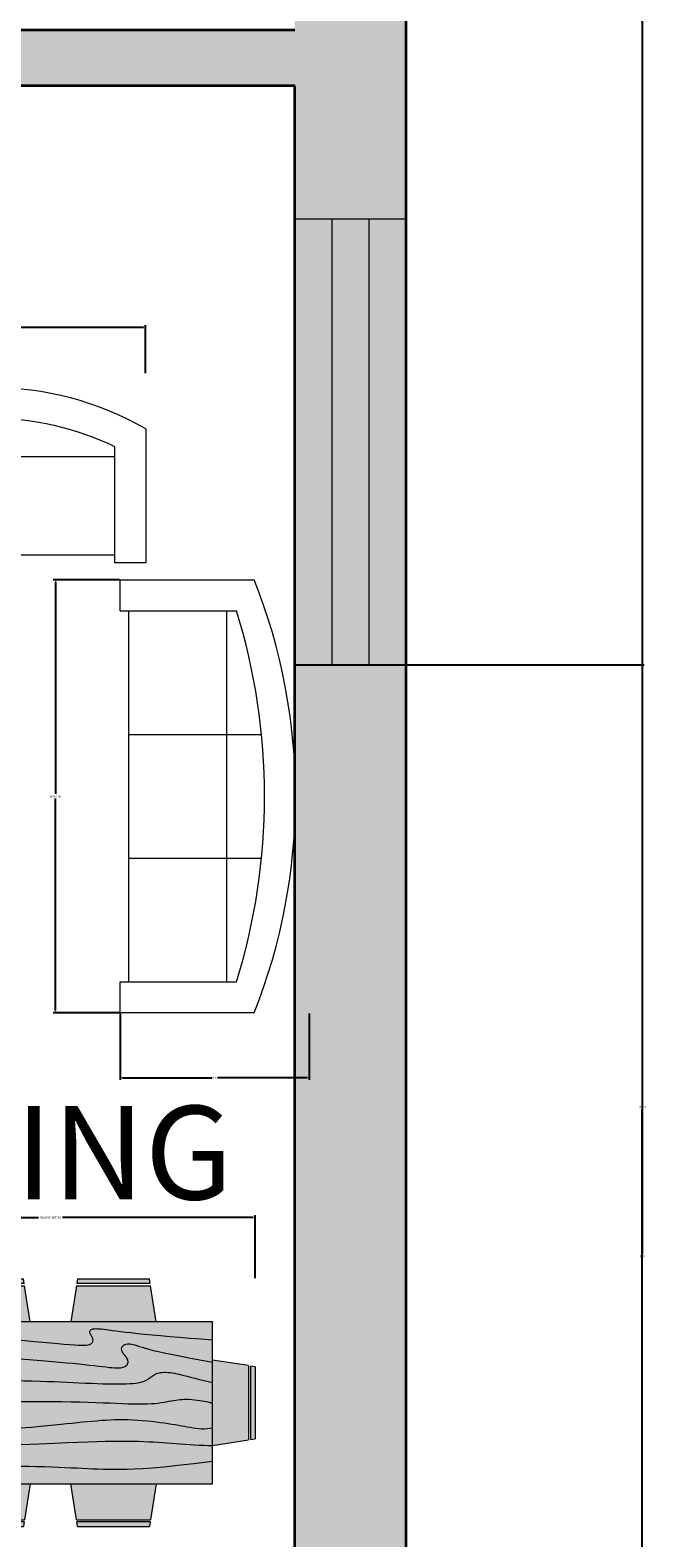
# Model space of a CAD drawing. Units: inches. Extents: x 857 to 1111, y 424 to 822.
# Tile 8 of 9: x 1062 to 1111, y 600 to 722. Entities that reach past the tile are written whole.
import ezdxf

# ---------------------------------------------------------------- set-up
doc = ezdxf.new("R2010")
doc.units = ezdxf.units.IN
for name, color, linetype, lineweight in [('A-ANNO-DIMS', 2, 'Continuous', 18), ('A-AREA-IDEN', 7, 'Continuous', 25), ('A-FURN', 8, 'Continuous', 18), ('A-FURN-PATT', 9, 'Continuous', 13), ('A-GLAZ', 4, 'Continuous', 18), ('A-GLAZ-PATT', 9, 'Continuous', 13), ('A-WALL', 7, 'Continuous', 35), ('A-WALL-PATT', 252, 'Continuous', 13)]:
    doc.layers.add(name, color=color, linetype=linetype, lineweight=lineweight)
doc.styles.get("Standard").update_dxf_attribs({"font": 'arial.ttf'})
doc.dimstyles.get("Standard").update_dxf_attribs({"dimtxt": 0.18, "dimasz": 0.18, "dimexe": 0.18, "dimexo": 0.0625, "dimgap": 0.09, "dimtad": 0, "dimtih": 1, "dimtoh": 1, "dimdec": 4, "dimzin": 0, "dimdsep": 46, "dimtxsty": 'Standard', "dimcen": 0.09, "dimadec": 0, "dimazin": 0, "dimtfac": 1, "dimtdec": 4, "dimtofl": 0, "dimtmove": 0, "dimatfit": 3, "dimfxl": 1, "dimtolj": 1, "dimtzin": 0, "dimarcsym": 0})

# ---------------------------------------------------------------- blocks, each defined once
blk = doc.blocks.new('Dining Set - 36 x 72 in.')
for p, q in [((-22, 27.5), (-22.1562, 26.50042)), ((-22, 27.5), (-6, 27.5)), ((-5.8437, 26.49966), (-6, 27.5)), ((6, 27.5), (5.8438, 26.50042)), ((6, 27.5), (22, 27.5)), ((22.1563, 26.49966), (22, 27.5)), ((-22.2343, 26.00059), (-23.4847, 17.99762)), ((-22.2304, 26), (-5.7608, 26)), ((-5.8416, 26.5), (-22.1534, 26.5)), ((-4.5152, 17.99762), (-5.7655, 25.99926)), ((5.7657, 26.00059), (4.5153, 17.99762)), ((5.7696, 26), (22.2392, 26)), ((22.1584, 26.5), (5.8466, 26.5)), ((23.4848, 17.99762), (22.2345, 25.99926)), ((36, 18), (-36, 18)), ((-36, 18), (-36, -18)), ((36, -18), (36, 18)), ((-45.5, 8), (-44.5004, 8.15617)), ((-45.5, 8), (-45.5, -8)), ((-44.5, -8.15843), (-44.5, 8.15338)), ((-44.0006, 8.23428), (-35.9976, 9.48474)), ((-44, 8.23041), (-44, -8.23915)), ((44.0006, 8.23428), (35.9976, 9.48474)), ((44, 8.23041), (44, -8.23915)), ((44.5, -8.15843), (44.5, 8.15338)), ((45.5, 8), (44.5005, 8.15617)), ((45.5, 8), (45.5, -8)), ((-44.4997, -8.15631), (-45.5, -8)), ((-35.9976, -9.48476), (-43.9993, -8.2345)), ((35.9976, -9.48476), (43.9993, -8.2345)), ((44.4997, -8.15631), (45.5, -8)), ((-36, -18), (36, -18)), ((-22.2343, -26.0006), (-23.4847, -17.99762)), ((-4.5152, -17.99762), (-5.7655, -25.99928)), ((5.7657, -26.0006), (4.5153, -17.99762)), ((23.4848, -17.99762), (22.2345, -25.99928)), ((-22.2304, -26), (-5.7608, -26)), ((-22, -27.5), (-22.1562, -26.50044)), ((-5.8416, -26.5), (-22.1534, -26.5)), ((-5.8437, -26.49967), (-6, -27.5)), ((5.7696, -26), (22.2392, -26)), ((6, -27.5), (5.8438, -26.50044)), ((22.1584, -26.5), (5.8466, -26.5)), ((22.1563, -26.49967), (22, -27.5)), ((-22, -27.5), (-6, -27.5)), ((6, -27.5), (22, -27.5))]:
    blk.add_line(p, q)
for points in [[(-36, 15), (-31.1772, 14.97754), (-26.8079, 14.91406), (-22.8538, 14.81543), (-19.276, 14.6875), (-16.0362, 14.53613), (-13.0957, 14.36718), (-10.4159, 14.18652), (-7.9583, 14), (-5.6904, 13.81315), (-3.6035, 13.63021), (-1.6954, 13.45508), (0.0365, 13.29166), (1.5945, 13.14388), (2.9811, 13.01562), (4.1988, 12.9108), (5.25, 12.83333), (6.1393, 12.78613), (6.8802, 12.76823), (7.4883, 12.77767), (7.9792, 12.8125), (8.3685, 12.87077), (8.6719, 12.95052), (8.9049, 13.0498), (9.0833, 13.16666), (9.2205, 13.29899), (9.3216, 13.44401), (9.3895, 13.59879), (9.4271, 13.76041), (9.4373, 13.92594), (9.4232, 14.09245), (9.3875, 14.257), (9.3333, 14.41666), (9.2638, 14.56917), (9.1836, 14.71484), (9.0975, 14.85465), (9.0104, 14.98958), (8.9272, 15.1206), (8.8529, 15.2487), (8.7922, 15.37483), (8.75, 15.5), (8.7305, 15.62467), (8.7344, 15.74739), (8.7617, 15.86621), (8.8125, 15.97916), (8.8867, 16.08431), (8.9844, 16.17968), (9.1055, 16.26334), (9.25, 16.33333), (9.4189, 16.38802), (9.6172, 16.42708), (9.8506, 16.45052), (10.125, 16.45833), (10.4463, 16.45052), (10.8203, 16.42708), (11.2529, 16.38802), (11.75, 16.33333), (12.3184, 16.26318), (12.9694, 16.17838), (13.7151, 16.07991), (14.5677, 15.96875), (15.5395, 15.84586), (16.6426, 15.71224), (17.8893, 15.56884), (19.2917, 15.41666), (20.859, 15.25667), (22.5879, 15.08984), (24.4721, 14.91715), (26.5052, 14.73958), (28.6809, 14.5581), (30.9929, 14.3737), (33.4347, 14.18733), (36, 14)], [(-36, 10), (-28.9766, 10.14274), (-23.1725, 10.20442), (-18.4241, 10.19775), (-14.5677, 10.13541), (-11.4399, 10.03011), (-8.877, 9.89453), (-6.7154, 9.74137), (-4.7917, 9.58333), (-2.9698, 9.43082), (-1.2246, 9.28515), (0.4415, 9.14534), (2.026, 9.01041), (3.5266, 8.87939), (4.9408, 8.7513), (6.266, 8.62516), (7.5, 8.5), (8.6411, 8.37549), (9.6914, 8.2539), (10.6538, 8.13818), (11.5312, 8.03125), (12.3267, 7.93603), (13.043, 7.85547), (13.6831, 7.79248), (14.25, 7.75), (14.7471, 7.7303), (15.1797, 7.73307), (15.5537, 7.75732), (15.875, 7.80208), (16.1494, 7.86637), (16.3828, 7.94922), (16.5811, 8.04964), (16.75, 8.16666), (16.8944, 8.29915), (17.0143, 8.44531), (17.1089, 8.60319), (17.1771, 8.77083), (17.218, 8.94629), (17.2305, 9.1276), (17.2137, 9.31282), (17.1667, 9.5), (17.0895, 9.6875), (16.987, 9.875), (16.8649, 10.0625), (16.7292, 10.25), (16.5856, 10.4375), (16.4401, 10.625), (16.2985, 10.8125), (16.1667, 11), (16.05, 11.18733), (15.9518, 11.3737), (15.8752, 11.5581), (15.8229, 11.73958), (15.798, 11.91715), (15.8034, 12.08984), (15.842, 12.25667), (15.9167, 12.41666), (16.0295, 12.56836), (16.1784, 12.70833), (16.3605, 12.83268), (16.5729, 12.9375), (16.8127, 13.01888), (17.0768, 13.07291), (17.3625, 13.0957), (17.6667, 13.08333), (17.9894, 13.03312), (18.3418, 12.94726), (18.7382, 12.82918), (19.1927, 12.68229), (19.7195, 12.51001), (20.3327, 12.31575), (21.0465, 12.10294), (21.875, 11.875), (22.8357, 11.63354), (23.959, 11.37304), (25.2786, 11.08618), (26.8282, 10.76562), (28.6414, 10.40405), (30.752, 9.99414), (33.1936, 9.52856), (36, 9)], [(-36, 5.5), (-30.7157, 5.3348), (-26.069, 5.20963), (-21.9946, 5.11767), (-18.4271, 5.05208), (-15.3009, 5.00602), (-12.5508, 4.97265), (-10.1112, 4.94515), (-7.9167, 4.91666), (-5.909, 4.88167), (-4.0586, 4.83984), (-2.3429, 4.79215), (-0.7396, 4.73958), (0.7739, 4.6831), (2.22, 4.6237), (3.6213, 4.56233), (5, 4.5), (6.373, 4.43782), (7.7344, 4.3776), (9.0723, 4.32129), (10.375, 4.27083), (11.6309, 4.22819), (12.8281, 4.19531), (13.9551, 4.17415), (15, 4.16666), (15.954, 4.17448), (16.819, 4.19791), (17.6001, 4.23698), (18.3021, 4.29166), (18.9299, 4.36198), (19.4883, 4.44791), (19.9823, 4.54948), (20.4167, 4.66666), (20.7969, 4.79899), (21.1302, 4.94401), (21.4245, 5.09879), (21.6875, 5.26041), (21.9271, 5.42594), (22.1511, 5.59245), (22.3672, 5.757), (22.5834, 5.91666), (22.8065, 6.06868), (23.0404, 6.21093), (23.2879, 6.34147), (23.5521, 6.45833), (23.8358, 6.55957), (24.142, 6.64323), (24.4735, 6.70735), (24.8334, 6.75), (25.2235, 6.76969), (25.642, 6.76692), (26.0858, 6.74267), (26.5521, 6.69791), (27.0379, 6.63362), (27.5404, 6.55078), (28.0565, 6.45036), (28.5834, 6.33333), (29.1242, 6.19987), (29.7071, 6.04687), (30.3661, 5.87044), (31.1354, 5.66666), (32.0493, 5.43164), (33.142, 5.16146), (34.4475, 4.85221), (36, 4.5)], [(-36, -1), (-30.7915, -0.6591), (-26.0195, -0.38216), (-21.6519, -0.16284), (-17.6563, 0.00521), (-14.0005, 0.12833), (-10.6523, 0.21289), (-7.5796, 0.26522), (-4.75, 0.29166), (-2.134, 0.29793), (0.2878, 0.28711), (2.5317, 0.26163), (4.6146, 0.22396), (6.5529, 0.17651), (8.3633, 0.12174), (10.0623, 0.06209), (11.6667, 0), (13.1899, -0.06201), (14.6341, -0.1211), (15.9982, -0.17432), (17.2813, -0.21875), (18.4823, -0.25147), (19.6003, -0.26953), (20.6343, -0.27002), (21.5834, -0.25), (22.4481, -0.20768), (23.2357, -0.14584), (23.9549, -0.06836), (24.6146, 0.02083), (25.2235, 0.11784), (25.7904, 0.21875), (26.3241, 0.31966), (26.8334, 0.41666), (27.3265, 0.50618), (27.8099, 0.58593), (28.2894, 0.65397), (28.7709, 0.70833), (29.2601, 0.74707), (29.763, 0.76823), (30.2855, 0.76985), (30.8334, 0.75), (31.4088, 0.70784), (31.9994, 0.64713), (32.589, 0.57275), (33.1615, 0.48958), (33.7008, 0.4025), (34.1908, 0.3164), (34.6153, 0.23616), (34.9584, 0.16666), (35.2099, 0.11165), (35.3848, 0.07031), (35.504, 0.04069), (35.5886, 0.02083), (35.6594, 0.00879), (35.7377, 0.0026), (35.8442, 0.00032), (36, 0)], [(-36, -6.5), (-27.1843, -6.31267), (-20.084, -6.1263), (-14.469, -5.9419), (-10.1094, -5.76042), (-6.7752, -5.58285), (-4.2363, -5.41016), (-2.2629, -5.24333), (-0.625, -5.08334), (0.8708, -4.93099), (2.2715, -4.78646), (3.5872, -4.64974), (4.8281, -4.52084), (6.0046, -4.39974), (7.127, -4.28646), (8.2053, -4.18099), (9.25, -4.08334), (10.2705, -3.99382), (11.2734, -3.91407), (12.2647, -3.84603), (13.25, -3.79167), (14.2354, -3.75293), (15.2266, -3.73177), (16.2295, -3.73015), (17.25, -3.75), (18.2912, -3.79248), (19.3451, -3.85547), (20.4009, -3.93604), (21.4479, -4.03125), (22.4754, -4.13819), (23.4727, -4.25391), (24.4289, -4.37549), (25.3334, -4.5), (26.1785, -4.62492), (26.9694, -4.74935), (27.7145, -4.87281), (28.4219, -4.99479), (29.1, -5.11483), (29.7572, -5.23242), (30.4016, -5.34709), (31.0417, -5.45834), (31.6837, -5.56437), (32.3262, -5.65821), (32.9658, -5.73153), (33.599, -5.77604), (34.2224, -5.78345), (34.8327, -5.74545), (35.4264, -5.65373), (36, -5.5)], [(-36, -10), (-26.4022, -9.81299), (-18.4675, -9.62891), (-11.9839, -9.45069), (-6.7396, -9.28125), (-2.5226, -9.12354), (0.8789, -8.98047), (3.6769, -8.85498), (6.0833, -8.75), (8.2767, -8.66765), (10.3021, -8.60677), (12.1712, -8.56543), (13.8958, -8.54167), (15.4876, -8.53353), (16.9583, -8.53907), (18.3197, -8.55632), (19.5834, -8.58334), (20.7616, -8.61841), (21.8685, -8.66081), (22.9188, -8.71004), (23.9271, -8.76563), (24.9081, -8.82707), (25.8763, -8.89388), (26.8465, -8.96558), (27.8334, -9.04167), (28.8474, -9.12118), (29.8828, -9.20117), (30.93, -9.27824), (31.9792, -9.34896), (33.0205, -9.40991), (34.0443, -9.45768), (35.0407, -9.48885), (36, -9.5)], [(-36, -14.5), (-30.0881, -14.33513), (-25.0332, -14.21224), (-20.7312, -14.12647), (-17.0781, -14.07292), (-13.97, -14.04671), (-11.3027, -14.04297), (-8.9724, -14.05681), (-6.875, -14.08334), (-4.9224, -14.11833), (-3.0905, -14.16016), (-1.3709, -14.20785), (0.2448, -14.26042), (1.7647, -14.3169), (3.1973, -14.3763), (4.5507, -14.43767), (5.8333, -14.5), (7.0554, -14.5621), (8.235, -14.62175), (9.3922, -14.67652), (10.5469, -14.72396), (11.7192, -14.76164), (12.929, -14.78711), (14.1965, -14.79794), (15.5417, -14.79167), (16.9933, -14.76424), (18.6152, -14.70508), (20.4804, -14.60197), (22.6615, -14.44271), (25.2312, -14.21509), (28.2624, -13.9069), (31.8277, -13.50594), (36, -13)]]:
    blk.add_lwpolyline(points)
blk = doc.blocks.new('Sofa - Roundback 7 ft.')
for p, q in [((-12.00002, -32.4421), (-12.00003, -6.5971)), ((11.99997, -32.4421), (11.99998, -6.5971)), ((-36.000027, -34), (-36.000027, -11.4696)), ((35.99998, -34), (35.99998, -11.4696)), ((-35.999844, -13.3819), (35.9998, -13.3819)), ((-36.000027, -32.4421), (35.99998, -32.4421))]:
    blk.add_line(p, q)
for points in [[(-36.000027, -34), (-42.000027, -34), (-42.000027, -8)], [(41.99998, -8), (41.99998, -34), (35.99998, -34)]]:
    blk.add_lwpolyline(points)
for centre, radius, start, end in [((0, -114.25), 114.25, 68.43141, 111.5686), ((-0.00001, -127.1968), 121.1968, 72.72033, 107.2797)]:
    blk.add_arc(centre, radius, start, end)
blk = doc.blocks.new('Sofa - Roundback Loveseat 5 ft.')
for p, q in [((0, -32.44198), (0, -5.99998)), ((-24, -33.99998), (-24, -11.46958)), ((24.00004, -33.99998), (24.00004, -11.46958)), ((-23.9998, -13.38178), (23.99986, -13.38178)), ((-24, -32.44198), (24.00004, -32.44198))]:
    blk.add_line(p, q)
for points in [[(-24, -33.99998), (-30, -33.99998), (-30, -7.99998)], [(30.00004, -7.99998), (30.00004, -33.99998), (24.00004, -33.99998)]]:
    blk.add_lwpolyline(points)
for centre, radius, start, end in [((0, -60.24998), 60.24998, 60.13715, 119.8628), ((0, -61.38438), 55.38444, 64.32083, 115.6792)]:
    blk.add_arc(centre, radius, start, end)
blk = doc.blocks.new('WIN-36IN-9IN-WALL')
for p, q in [((3, 36), (3, 0)), ((6, 0), (6, 36))]:
    blk.add_line(p, q)
blk.add_lwpolyline([(0, 36), (0, 0), (9, 0), (9, 36)], close=True)
blk = doc.blocks.new('*D30')
at = {"layer": 'A-ANNO-DIMS', "color": 0, "lineweight": -2, "transparency": 16777216}
for p, q in [((1046.89, 621.08), (1046.89, 626.16)), ((1047.07, 625.98), (1062.45, 625.98)), ((1079.77, 625.98), (1064.39, 625.98)), ((1079.95, 621.08), (1079.95, 626.16))]:
    blk.add_line(p, q, dxfattribs=at)
at = {"layer": 'A-ANNO-DIMS', "color": 0, "transparency": 16777216}
for points in [[(1047.07, 626.01), (1047.07, 625.95), (1046.89, 625.98)], [(1079.77, 626.01), (1079.77, 625.95), (1079.95, 625.98)]]:
    blk.add_solid(points, dxfattribs=at)
at = {"layer": 'Defpoints', "color": 0, "transparency": 16777216}
for p in [(1079.95, 625.98), (1046.89, 621.02), (1079.95, 621.02)]:
    blk.add_point(p, dxfattribs=at)
at = {"layer": 'A-ANNO-DIMS', "color": 0, "transparency": 16777216, "insert": (1063.42, 625.98), "char_height": 0.18, "attachment_point": 5}
blk.add_mtext('\\A1;DINING SET 33', dxfattribs=at)
blk = doc.blocks.new('*D34')
at = {"layer": 'A-ANNO-DIMS', "color": 0, "lineweight": -2, "transparency": 16777216}
for p, q in [((1068.99, 677.48), (1063.63, 677.48)), ((1063.81, 677.3), (1063.81, 660.18)), ((1063.81, 642.69), (1063.81, 659.81)), ((1068.99, 642.51), (1063.63, 642.51))]:
    blk.add_line(p, q, dxfattribs=at)
at = {"layer": 'A-ANNO-DIMS', "color": 0, "transparency": 16777216}
for points in [[(1063.78, 677.3), (1063.84, 677.3), (1063.81, 677.48)], [(1063.78, 642.69), (1063.84, 642.69), (1063.81, 642.51)]]:
    blk.add_solid(points, dxfattribs=at)
at = {"layer": 'Defpoints', "color": 0, "transparency": 16777216}
for p in [(1069.05, 677.48), (1063.81, 642.51), (1069.05, 642.51)]:
    blk.add_point(p, dxfattribs=at)
at = {"layer": 'A-ANNO-DIMS', "color": 0, "transparency": 16777216, "insert": (1063.81, 659.99), "char_height": 0.18, "attachment_point": 5}
blk.add_mtext('\\A1;SOFA 35', dxfattribs=at)
blk = doc.blocks.new('*D35')
at = {"layer": 'A-ANNO-DIMS', "color": 0, "lineweight": -2, "transparency": 16777216}
for p, q in [((1069.05, 642.45), (1069.05, 637.09)), ((1084.31, 642.45), (1084.31, 637.09)), ((1069.23, 637.27), (1076.47, 637.27)), ((1084.13, 637.27), (1076.9, 637.27))]:
    blk.add_line(p, q, dxfattribs=at)
at = {"layer": 'A-ANNO-DIMS', "color": 0, "transparency": 16777216}
for points in [[(1069.23, 637.3), (1069.23, 637.24), (1069.05, 637.27)], [(1084.13, 637.3), (1084.13, 637.24), (1084.31, 637.27)]]:
    blk.add_solid(points, dxfattribs=at)
at = {"layer": 'Defpoints', "color": 0, "transparency": 16777216}
for p in [(1069.05, 642.51), (1084.31, 642.51), (1084.31, 637.27)]:
    blk.add_point(p, dxfattribs=at)
at = {"layer": 'A-ANNO-DIMS', "color": 0, "transparency": 16777216, "insert": (1076.68, 637.27), "char_height": 0.18, "attachment_point": 5}
blk.add_mtext('\\A1;15', dxfattribs=at)
blk = doc.blocks.new('*D36')
at = {"layer": 'A-ANNO-DIMS', "color": 0, "lineweight": -2, "transparency": 16777216}
for p, q in [((1046.13, 694.16), (1046.13, 698.03)), ((1046.31, 697.85), (1057.7, 697.85)), ((1070.92, 697.85), (1059.53, 697.85)), ((1071.1, 694.16), (1071.1, 698.03))]:
    blk.add_line(p, q, dxfattribs=at)
at = {"layer": 'A-ANNO-DIMS', "color": 0, "transparency": 16777216}
for points in [[(1046.31, 697.88), (1046.31, 697.82), (1046.13, 697.85)], [(1070.92, 697.88), (1070.92, 697.82), (1071.1, 697.85)]]:
    blk.add_solid(points, dxfattribs=at)
at = {"layer": 'Defpoints', "color": 0, "transparency": 16777216}
for p in [(1071.1, 697.85), (1046.13, 694.1), (1071.1, 694.1)]:
    blk.add_point(p, dxfattribs=at)
at = {"layer": 'A-ANNO-DIMS', "color": 0, "transparency": 16777216, "insert": (1058.62, 697.85), "char_height": 0.18, "attachment_point": 5}
blk.add_mtext('\\A1;LOVESEAT 25', dxfattribs=at)
blk = doc.blocks.new('*D45')
at = {"layer": 'A-ANNO-DIMS', "color": 0, "lineweight": -2, "transparency": 16777216}
for p, q in [((1092.2, 802.86), (1111.37, 802.86)), ((1111.19, 802.68), (1111.19, 623.04)), ((1111.19, 443.04), (1111.19, 622.67)), ((1092.2, 442.86), (1111.37, 442.86))]:
    blk.add_line(p, q, dxfattribs=at)
at = {"layer": 'A-ANNO-DIMS', "color": 0, "transparency": 16777216}
for points in [[(1111.16, 802.68), (1111.22, 802.68), (1111.19, 802.86)], [(1111.16, 443.04), (1111.22, 443.04), (1111.19, 442.86)]]:
    blk.add_solid(points, dxfattribs=at)
at = {"layer": 'Defpoints', "color": 0, "transparency": 16777216}
for p in [(1092.14, 802.86), (1111.19, 802.86), (1092.14, 442.86)]:
    blk.add_point(p, dxfattribs=at)
at = {"layer": 'A-ANNO-DIMS', "color": 0, "transparency": 16777216, "insert": (1111.19, 622.86), "char_height": 0.18, "attachment_point": 5}
blk.add_mtext('\\A1;360', dxfattribs=at)
blk = doc.blocks.new('*D55')
at = {"layer": 'A-ANNO-DIMS', "color": 0, "lineweight": -2, "transparency": 16777216}
for p, q in [((1053.97, 717.29), (1053.97, 423.63)), ((1083.14, 717.29), (1083.14, 423.63)), ((1054.15, 423.81), (1068.09, 423.81)), ((1082.96, 423.81), (1069.02, 423.81))]:
    blk.add_line(p, q, dxfattribs=at)
at = {"layer": 'A-ANNO-DIMS', "color": 0, "transparency": 16777216}
for points in [[(1054.15, 423.84), (1054.15, 423.78), (1053.97, 423.81)], [(1082.96, 423.84), (1082.96, 423.78), (1083.14, 423.81)]]:
    blk.add_solid(points, dxfattribs=at)
at = {"layer": 'Defpoints', "color": 0, "transparency": 16777216}
for p in [(1053.97, 717.36), (1083.14, 717.36), (1083.14, 423.81)]:
    blk.add_point(p, dxfattribs=at)
at = {"layer": 'A-ANNO-DIMS', "color": 0, "transparency": 16777216, "insert": (1068.55, 423.81), "char_height": 0.18, "attachment_point": 5}
blk.add_mtext('\\A1;29.165', dxfattribs=at)
blk = doc.blocks.new('*D61')
at = {"layer": 'A-ANNO-DIMS', "color": 0, "lineweight": -2, "transparency": 16777216}
for p, q in [((1083.2, 670.61), (1111.37, 670.61)), ((1111.19, 670.43), (1111.19, 635.08)), ((1111.19, 599.37), (1111.19, 634.72)), ((1083.2, 599.19), (1111.37, 599.19))]:
    blk.add_line(p, q, dxfattribs=at)
at = {"layer": 'A-ANNO-DIMS', "color": 0, "transparency": 16777216}
for points in [[(1111.16, 670.43), (1111.22, 670.43), (1111.19, 670.61)], [(1111.16, 599.37), (1111.22, 599.37), (1111.19, 599.19)]]:
    blk.add_solid(points, dxfattribs=at)
at = {"layer": 'Defpoints', "color": 0, "transparency": 16777216}
for p in [(1083.14, 670.61), (1111.19, 670.61), (1083.14, 599.19)]:
    blk.add_point(p, dxfattribs=at)
at = {"layer": 'A-ANNO-DIMS', "color": 0, "transparency": 16777216, "insert": (1111.19, 634.9), "char_height": 0.18, "attachment_point": 5}
blk.add_mtext('\\A1;71.41', dxfattribs=at)

msp = doc.modelspace()

# ---------------------------------------------------------------- hatches: boundary and pattern name
at = {"layer": 'A-FURN-PATT'}
h = msp.add_hatch(color=256, dxfattribs=at)
h.dxf.hatch_style = 1
h.paths.add_polyline_path([(1071.4125, 621.0178), (1065.599, 621.0178), (1065.5422, 620.6545), (1071.4693, 620.6545)])
h.paths.add_polyline_path([(1071.4977, 620.4728), (1065.5138, 620.4728), (1065.0596, 617.566), (1071.9519, 617.566)])
h.paths.add_polyline_path([(1061.324, 620.4728), (1055.3401, 620.4728), (1054.8859, 617.566), (1061.7782, 617.566)])
h.paths.add_polyline_path([(1061.2388, 621.0178), (1055.4253, 621.0178), (1055.3685, 620.6545), (1061.2956, 620.6545)])
h.paths.add_polyline_path([(1050.3384, 614.4719), (1047.4316, 614.0177), (1047.4316, 608.0338), (1050.3384, 607.5797)])
h.paths.add_polyline_path([(1047.25, 613.9893), (1046.8866, 613.9326), (1046.8866, 608.119), (1047.25, 608.0622)])
h.paths.add_polyline_path([(1061.7782, 604.4855), (1054.8859, 604.4855), (1055.3401, 601.5788), (1061.324, 601.5788)])
h.paths.add_polyline_path([(1061.2956, 601.3971), (1055.3685, 601.3971), (1055.4253, 601.0337), (1061.2388, 601.0337)])
h.paths.add_polyline_path([(1071.4693, 601.3971), (1065.5422, 601.3971), (1065.599, 601.0337), (1071.4125, 601.0337)])
h.paths.add_polyline_path([(1071.9519, 604.4855), (1065.0596, 604.4855), (1065.5138, 601.5788), (1071.4977, 601.5788)])
h.paths.add_polyline_path([(1079.4062, 614.0177), (1076.4994, 614.4719), (1076.4994, 607.5797), (1079.4062, 608.0338)])
h.paths.add_polyline_path([(1079.9512, 613.9326), (1079.5878, 613.9893), (1079.5878, 608.0622), (1079.9512, 608.119)])
h = msp.add_hatch(color=256, dxfattribs=at)
h.dxf.hatch_style = 1
h.paths.add_polyline_path([(1066.6626, 616.5198), (1066.6356, 616.5664), (1066.6135, 616.6122), (1066.5982, 616.6577), (1066.5911, 616.703), (1066.5925, 616.7476), (1066.6024, 616.7907), (1066.6209, 616.8318), (1066.6478, 616.87), (1066.6833, 616.9046), (1066.7273, 616.935), (1066.7798, 616.9605), (1066.8412, 616.9803), (1066.9133, 616.9945), (1066.9981, 617.003), (1067.0978, 617.0059), (1067.2145, 617.003), (1067.3504, 616.9945), (1067.5076, 616.9803), (1067.6882, 616.9605), (1067.8947, 616.935), (1068.1313, 616.9042), (1068.4022, 616.8684), (1068.712, 616.828), (1069.0651, 616.7833), (1069.4659, 616.7348), (1069.9189, 616.6827), (1070.4285, 616.6274), (1070.9979, 616.5692), (1071.6261, 616.5086), (1072.3108, 616.4459), (1073.0495, 616.3814), (1073.84, 616.3154), (1074.6801, 616.2484), (1075.5673, 616.1807), (1076.4994, 616.1126), (1076.4994, 617.566), (1050.3384, 617.566), (1050.3384, 616.476), (1052.0907, 616.4678), (1053.6783, 616.4448), (1055.115, 616.4089), (1056.415, 616.3624), (1057.5922, 616.3074), (1058.6606, 616.2461), (1059.6343, 616.1804), (1060.5273, 616.1126), (1061.3513, 616.0448), (1062.1096, 615.9783), (1062.8029, 615.9146), (1063.4322, 615.8553), (1063.9982, 615.8016), (1064.5021, 615.755), (1064.9445, 615.7169), (1065.3265, 615.6887), (1065.6496, 615.6716), (1065.9188, 615.6651), (1066.1397, 615.6685), (1066.3181, 615.6812), (1066.4596, 615.7023), (1066.5698, 615.7313), (1066.6545, 615.7674), (1066.7193, 615.8099), (1066.7691, 615.8579), (1066.8059, 615.9106), (1066.8305, 615.9669), (1066.8442, 616.0256), (1066.8479, 616.0857), (1066.8428, 616.1462), (1066.8298, 616.206), (1066.8101, 616.264), (1066.7849, 616.3194), (1066.7557, 616.3724), (1066.7244, 616.4232), (1066.6928, 616.4722)])
h.paths.add_polyline_path([(1069.2432, 615.5925), (1069.2973, 615.6433), (1069.3634, 615.6885), (1069.4406, 615.7266), (1069.5277, 615.7562), (1069.6237, 615.7758), (1069.7275, 615.7841), (1069.838, 615.7796), (1069.9553, 615.7613), (1070.0833, 615.7301), (1070.2274, 615.6872), (1070.3925, 615.6339), (1070.5839, 615.5713), (1070.8067, 615.5007), (1071.0661, 615.4234), (1071.3671, 615.3405), (1071.7162, 615.2528), (1072.1243, 615.1581), (1072.6038, 615.0539), (1073.1668, 614.9374), (1073.8257, 614.8061), (1074.5925, 614.6571), (1075.4797, 614.488), (1076.4994, 614.2959), (1076.4994, 616.1126), (1075.5673, 616.1807), (1074.6801, 616.2484), (1073.84, 616.3154), (1073.0495, 616.3814), (1072.3108, 616.4459), (1071.6261, 616.5086), (1070.9979, 616.5692), (1070.4285, 616.6274), (1069.9189, 616.6827), (1069.4659, 616.7348), (1069.0651, 616.7833), (1068.712, 616.828), (1068.4022, 616.8684), (1068.1313, 616.9042), (1067.8947, 616.935), (1067.6882, 616.9605), (1067.5076, 616.9803), (1067.3504, 616.9945), (1067.2145, 617.003), (1067.0978, 617.0059), (1066.9981, 617.003), (1066.9133, 616.9945), (1066.8412, 616.9803), (1066.7798, 616.9605), (1066.7273, 616.935), (1066.6833, 616.9046), (1066.6478, 616.87), (1066.6209, 616.8318), (1066.6024, 616.7907), (1066.5925, 616.7476), (1066.5911, 616.703), (1066.5982, 616.6577), (1066.6135, 616.6122), (1066.6356, 616.5664), (1066.6626, 616.5198), (1066.6928, 616.4722), (1066.7244, 616.4232), (1066.7557, 616.3724), (1066.7849, 616.3194), (1066.8101, 616.264), (1066.8298, 616.206), (1066.8428, 616.1462), (1066.8479, 616.0857), (1066.8442, 616.0256), (1066.8305, 615.9669), (1066.8059, 615.9106), (1066.7691, 615.8579), (1066.7193, 615.8099), (1066.6545, 615.7674), (1066.5698, 615.7313), (1066.4596, 615.7023), (1066.3181, 615.6812), (1066.1397, 615.6685), (1065.9188, 615.6651), (1065.6496, 615.6716), (1065.3265, 615.6887), (1064.9445, 615.7169), (1064.5021, 615.755), (1063.9982, 615.8016), (1063.4322, 615.8553), (1062.8029, 615.9146), (1062.1096, 615.9783), (1061.3513, 616.0448), (1060.5273, 616.1126), (1059.6343, 616.1804), (1058.6606, 616.2461), (1057.5922, 616.3074), (1056.415, 616.3624), (1055.115, 616.4089), (1053.6783, 616.4448), (1052.0907, 616.4678), (1050.3384, 616.476), (1050.3384, 614.6593), (1052.8903, 614.7111), (1054.9992, 614.7335), (1056.7245, 614.7311), (1058.1258, 614.7085), (1059.2622, 614.6702), (1060.1935, 614.6209), (1060.9789, 614.5653), (1061.6778, 614.5079), (1062.3398, 614.4524), (1062.9739, 614.3995), (1063.5793, 614.3487), (1064.155, 614.2997), (1064.7003, 614.2521), (1065.2141, 614.2055), (1065.6956, 614.1597), (1066.144, 614.1142), (1066.5586, 614.069), (1066.9402, 614.0248), (1067.2899, 613.9828), (1067.6087, 613.9439), (1067.8978, 613.9093), (1068.158, 613.88), (1068.3906, 613.8572), (1068.5966, 613.8417), (1068.7772, 613.8346), (1068.9344, 613.8356), (1069.0703, 613.8444), (1069.187, 613.8606), (1069.2867, 613.884), (1069.3715, 613.9141), (1069.4436, 613.9506), (1069.5049, 613.9931), (1069.5574, 614.0413), (1069.601, 614.0944), (1069.6354, 614.1517), (1069.6601, 614.2126), (1069.675, 614.2764), (1069.6795, 614.3423), (1069.6734, 614.4096), (1069.6564, 614.4776), (1069.6283, 614.5457), (1069.5911, 614.6138), (1069.5467, 614.682), (1069.4974, 614.7501), (1069.4452, 614.8182), (1069.3923, 614.8863), (1069.3409, 614.9545), (1069.293, 615.0226), (1069.2506, 615.0907), (1069.2149, 615.1584), (1069.1871, 615.2254), (1069.1681, 615.2913), (1069.159, 615.3558), (1069.161, 615.4186), (1069.175, 615.4792), (1069.2022, 615.5373)])
h.paths.add_polyline_path([(1076.4994, 614.2959), (1075.4797, 614.488), (1074.5925, 614.6571), (1073.8257, 614.8061), (1073.1668, 614.9374), (1072.6038, 615.0539), (1072.1243, 615.1581), (1071.7162, 615.2528), (1071.3671, 615.3405), (1071.0661, 615.4234), (1070.8067, 615.5007), (1070.5839, 615.5713), (1070.3925, 615.6339), (1070.2274, 615.6872), (1070.0833, 615.7301), (1069.9553, 615.7613), (1069.838, 615.7796), (1069.7275, 615.7841), (1069.6237, 615.7758), (1069.5277, 615.7562), (1069.4406, 615.7266), (1069.3634, 615.6885), (1069.2973, 615.6433), (1069.2432, 615.5925), (1069.2022, 615.5373), (1069.175, 615.4792), (1069.161, 615.4186), (1069.159, 615.3558), (1069.1681, 615.2913), (1069.1871, 615.2254), (1069.2149, 615.1584), (1069.2506, 615.0907), (1069.293, 615.0226), (1069.3409, 614.9545), (1069.3923, 614.8863), (1069.4452, 614.8182), (1069.4974, 614.7501), (1069.5467, 614.682), (1069.5911, 614.6138), (1069.6283, 614.5457), (1069.6564, 614.4776), (1069.6734, 614.4096), (1069.6795, 614.3423), (1069.675, 614.2764), (1069.6601, 614.2126), (1069.6354, 614.1517), (1069.601, 614.0944), (1069.5574, 614.0413), (1069.5049, 613.9931), (1069.4436, 613.9506), (1069.3715, 613.9141), (1069.2867, 613.884), (1069.187, 613.8606), (1069.0703, 613.8444), (1068.9344, 613.8356), (1068.7772, 613.8346), (1068.5966, 613.8417), (1068.3906, 613.8572), (1068.158, 613.88), (1067.8978, 613.9093), (1067.6087, 613.9439), (1067.2899, 613.9828), (1066.9402, 614.0248), (1066.5586, 614.069), (1066.144, 614.1142), (1065.6956, 614.1597), (1065.2141, 614.2055), (1064.7003, 614.2521), (1064.155, 614.2997), (1063.5793, 614.3487), (1062.9739, 614.3995), (1062.3398, 614.4524), (1061.6778, 614.5079), (1060.9789, 614.5653), (1060.1935, 614.6209), (1059.2622, 614.6702), (1058.1258, 614.7085), (1056.7245, 614.7311), (1054.9992, 614.7335), (1052.8903, 614.7111), (1050.3384, 614.6593), (1050.3384, 613.0242), (1052.2584, 612.9642), (1053.9468, 612.9187), (1055.4272, 612.8853), (1056.7235, 612.8614), (1057.8594, 612.8447), (1058.8586, 612.8326), (1059.745, 612.8226), (1060.5424, 612.8122), (1061.2719, 612.7995), (1061.9442, 612.7843), (1062.5676, 612.767), (1063.1502, 612.7479), (1063.7001, 612.7274), (1064.2255, 612.7058), (1064.7347, 612.6835), (1065.2356, 612.6608), (1065.7345, 612.6383), (1066.2292, 612.6164), (1066.7153, 612.5959), (1067.1886, 612.5776), (1067.6449, 612.5621), (1068.0799, 612.5501), (1068.4894, 612.5425), (1068.8691, 612.5397), (1069.2157, 612.5426), (1069.53, 612.5511), (1069.8138, 612.5653), (1070.0689, 612.5851), (1070.297, 612.6107), (1070.4999, 612.6419), (1070.6794, 612.6788), (1070.8372, 612.7214), (1070.9754, 612.7695), (1071.0965, 612.8222), (1071.2034, 612.8784), (1071.299, 612.9371), (1071.386, 612.9973), (1071.4674, 613.0578), (1071.5459, 613.1176), (1071.6245, 613.1756), (1071.7056, 613.2308), (1071.7905, 613.2825), (1071.8805, 613.3299), (1071.9765, 613.3724), (1072.0796, 613.4092), (1072.1908, 613.4396), (1072.3113, 613.4629), (1072.442, 613.4784), (1072.5838, 613.4855), (1072.7358, 613.4845), (1072.8971, 613.4757), (1073.0665, 613.4595), (1073.243, 613.4361), (1073.4256, 613.406), (1073.6131, 613.3695), (1073.8046, 613.327), (1074.0011, 613.2785), (1074.2129, 613.2229), (1074.4523, 613.1588), (1074.7318, 613.0847), (1075.0639, 612.9994), (1075.4609, 612.9012), (1075.9353, 612.7888), (1076.4994, 612.6608)])
h.paths.add_polyline_path([(1076.4994, 612.6608), (1075.9353, 612.7888), (1075.4609, 612.9012), (1075.0639, 612.9994), (1074.7318, 613.0847), (1074.4523, 613.1588), (1074.2129, 613.2229), (1074.0011, 613.2785), (1073.8046, 613.327), (1073.6131, 613.3695), (1073.4256, 613.406), (1073.243, 613.4361), (1073.0665, 613.4595), (1072.8971, 613.4757), (1072.7358, 613.4845), (1072.5838, 613.4855), (1072.442, 613.4784), (1072.3113, 613.4629), (1072.1908, 613.4396), (1072.0796, 613.4092), (1071.9765, 613.3724), (1071.8805, 613.3299), (1071.7905, 613.2825), (1071.7056, 613.2308), (1071.6245, 613.1756), (1071.5459, 613.1176), (1071.4674, 613.0578), (1071.386, 612.9973), (1071.299, 612.9371), (1071.2034, 612.8784), (1071.0965, 612.8222), (1070.9754, 612.7695), (1070.8372, 612.7214), (1070.6794, 612.6788), (1070.4999, 612.6419), (1070.297, 612.6107), (1070.0689, 612.5851), (1069.8138, 612.5653), (1069.53, 612.5511), (1069.2157, 612.5426), (1068.8691, 612.5397), (1068.4894, 612.5425), (1068.0799, 612.5501), (1067.6449, 612.5621), (1067.1886, 612.5776), (1066.7153, 612.5959), (1066.2292, 612.6164), (1065.7345, 612.6383), (1065.2356, 612.6608), (1064.7347, 612.6835), (1064.2255, 612.7058), (1063.7001, 612.7274), (1063.1502, 612.7479), (1062.5676, 612.767), (1061.9442, 612.7843), (1061.2719, 612.7995), (1060.5424, 612.8122), (1059.745, 612.8226), (1058.8586, 612.8326), (1057.8594, 612.8447), (1056.7235, 612.8614), (1055.4272, 612.8853), (1053.9468, 612.9187), (1052.2584, 612.9642), (1050.3384, 613.0242), (1050.3384, 610.6624), (1052.2309, 610.7863), (1053.9648, 610.8869), (1055.5517, 610.9666), (1057.0035, 611.0277), (1058.3319, 611.0724), (1059.5484, 611.1031), (1060.6649, 611.1222), (1061.693, 611.1318), (1062.6435, 611.134), (1063.5235, 611.1301), (1064.3388, 611.1208), (1065.0956, 611.1072), (1065.7999, 611.0899), (1066.4577, 611.07), (1067.075, 611.0483), (1067.6579, 611.0258), (1068.2114, 611.0033), (1068.7361, 610.9818), (1069.2318, 610.9624), (1069.698, 610.9463), (1070.1344, 610.9344), (1070.5406, 610.9279), (1070.9163, 610.9277), (1071.2612, 610.9349), (1071.5753, 610.9503), (1071.8615, 610.9728), (1072.1228, 611.0009), (1072.3625, 611.0334), (1072.5838, 611.0686), (1072.7898, 611.1053), (1072.9837, 611.1419), (1073.1687, 611.1772), (1073.3479, 611.2097), (1073.5235, 611.2387), (1073.6978, 611.2634), (1073.8727, 611.2832), (1074.0505, 611.2972), (1074.2332, 611.3049), (1074.423, 611.3055), (1074.6221, 611.2983), (1074.8312, 611.283), (1075.0458, 611.2609), (1075.26, 611.2339), (1075.468, 611.2037), (1075.664, 611.172), (1075.842, 611.1407), (1075.9963, 611.1116), (1076.1209, 611.0863), (1076.2123, 611.0664), (1076.2758, 611.0513), (1076.3192, 611.0406), (1076.3499, 611.0334), (1076.3756, 611.029), (1076.4041, 611.0267), (1076.4428, 611.0259), (1076.4994, 611.0258)])
h.paths.add_polyline_path([(1076.4994, 611.0258), (1076.4428, 611.0259), (1076.4041, 611.0267), (1076.3756, 611.029), (1076.3499, 611.0334), (1076.3192, 611.0406), (1076.2758, 611.0513), (1076.2123, 611.0664), (1076.1209, 611.0863), (1075.9963, 611.1116), (1075.842, 611.1407), (1075.664, 611.172), (1075.468, 611.2037), (1075.26, 611.2339), (1075.0458, 611.2609), (1074.8312, 611.283), (1074.6221, 611.2983), (1074.423, 611.3055), (1074.2332, 611.3049), (1074.0505, 611.2972), (1073.8727, 611.2832), (1073.6978, 611.2634), (1073.5235, 611.2387), (1073.3479, 611.2097), (1073.1687, 611.1772), (1072.9837, 611.1419), (1072.7898, 611.1053), (1072.5838, 611.0686), (1072.3625, 611.0334), (1072.1228, 611.0009), (1071.8615, 610.9728), (1071.5753, 610.9503), (1071.2612, 610.9349), (1070.9163, 610.9277), (1070.5406, 610.9279), (1070.1344, 610.9344), (1069.698, 610.9463), (1069.2318, 610.9624), (1068.7361, 610.9818), (1068.2114, 611.0033), (1067.6579, 611.0258), (1067.075, 611.0483), (1066.4577, 611.07), (1065.7999, 611.0899), (1065.0956, 611.1072), (1064.3388, 611.1208), (1063.5235, 611.1301), (1062.6435, 611.134), (1061.693, 611.1318), (1060.6649, 611.1222), (1059.5484, 611.1031), (1058.3319, 611.0724), (1057.0035, 611.0277), (1055.5517, 610.9666), (1053.9648, 610.8869), (1052.2309, 610.7863), (1050.3384, 610.6624), (1050.3384, 608.664), (1053.5416, 608.7321), (1056.1214, 608.7998), (1058.1616, 608.8668), (1059.7457, 608.9328), (1060.9571, 608.9973), (1061.8796, 609.06), (1062.5967, 609.1206), (1063.1918, 609.1788), (1063.7353, 609.2341), (1064.2442, 609.2866), (1064.7223, 609.3363), (1065.1732, 609.3832), (1065.6006, 609.4272), (1066.0085, 609.4683), (1066.4003, 609.5066), (1066.7798, 609.5421), (1067.1506, 609.5746), (1067.515, 609.6036), (1067.8752, 609.6283), (1068.2332, 609.6481), (1068.5913, 609.6622), (1068.9514, 609.6699), (1069.3158, 609.6704), (1069.6866, 609.6632), (1070.0649, 609.6478), (1070.4479, 609.6249), (1070.8315, 609.5956), (1071.2119, 609.561), (1071.5853, 609.5222), (1071.9476, 609.4801), (1072.2951, 609.436), (1072.6237, 609.3907), (1072.9308, 609.3453), (1073.2181, 609.3001), (1073.4889, 609.2553), (1073.7459, 609.2109), (1073.9923, 609.1673), (1074.2311, 609.1246), (1074.4652, 609.0829), (1074.6978, 609.0425), (1074.9311, 609.004), (1075.1645, 608.9699), (1075.3969, 608.9433), (1075.627, 608.9271), (1075.8535, 608.9244), (1076.0752, 608.9382), (1076.291, 608.9715), (1076.4994, 609.0274)])
h.paths.add_polyline_path([(1076.4994, 609.0274), (1076.291, 608.9715), (1076.0752, 608.9382), (1075.8535, 608.9244), (1075.627, 608.9271), (1075.3969, 608.9433), (1075.1645, 608.9699), (1074.9311, 609.004), (1074.6978, 609.0425), (1074.4652, 609.0829), (1074.2311, 609.1246), (1073.9923, 609.1673), (1073.7459, 609.2109), (1073.4889, 609.2553), (1073.2181, 609.3001), (1072.9308, 609.3453), (1072.6237, 609.3907), (1072.2951, 609.436), (1071.9476, 609.4801), (1071.5853, 609.5222), (1071.2119, 609.561), (1070.8315, 609.5956), (1070.4479, 609.6249), (1070.0649, 609.6478), (1069.6866, 609.6632), (1069.3158, 609.6704), (1068.9514, 609.6699), (1068.5913, 609.6622), (1068.2332, 609.6481), (1067.8752, 609.6283), (1067.515, 609.6036), (1067.1506, 609.5746), (1066.7798, 609.5421), (1066.4003, 609.5066), (1066.0085, 609.4683), (1065.6006, 609.4272), (1065.1732, 609.3832), (1064.7223, 609.3363), (1064.2442, 609.2866), (1063.7353, 609.2341), (1063.1918, 609.1788), (1062.5967, 609.1206), (1061.8796, 609.06), (1060.9571, 608.9973), (1059.7457, 608.9328), (1058.1616, 608.8668), (1056.1214, 608.7998), (1053.5416, 608.7321), (1050.3384, 608.664), (1050.3384, 607.3923), (1053.8257, 607.4603), (1056.7088, 607.5272), (1059.0646, 607.5919), (1060.9701, 607.6535), (1062.5023, 607.7108), (1063.7382, 607.7628), (1064.7549, 607.8084), (1065.6292, 607.8465), (1066.4262, 607.8764), (1067.1621, 607.8985), (1067.8413, 607.9136), (1068.4679, 607.9222), (1069.0463, 607.9252), (1069.5806, 607.9231), (1070.0753, 607.9169), (1070.5345, 607.9071), (1070.9626, 607.8943), (1071.3647, 607.8789), (1071.7464, 607.861), (1072.1127, 607.8408), (1072.4692, 607.8185), (1072.821, 607.7942), (1073.1735, 607.7682), (1073.5321, 607.7405), (1073.9005, 607.7116), (1074.2767, 607.6826), (1074.6572, 607.6546), (1075.0384, 607.6289), (1075.4168, 607.6067), (1075.7888, 607.5894), (1076.1508, 607.578), (1076.4994, 607.574)])
h.paths.add_polyline_path([(1076.4994, 606.3023), (1074.9834, 606.1184), (1073.6879, 605.9728), (1072.5866, 605.8608), (1071.6529, 605.7781), (1070.8604, 605.7202), (1070.1827, 605.6827), (1069.5934, 605.6612), (1069.0659, 605.6513), (1068.5771, 605.649), (1068.1166, 605.6529), (1067.677, 605.6622), (1067.2511, 605.6759), (1066.8315, 605.6931), (1066.4111, 605.713), (1065.9824, 605.7347), (1065.5384, 605.7573), (1065.0724, 605.7799), (1064.5806, 605.8022), (1064.0601, 605.8238), (1063.5078, 605.8443), (1062.9208, 605.8634), (1062.296, 605.8807), (1061.6304, 605.8959), (1060.9209, 605.9086), (1060.1588, 605.9183), (1059.3121, 605.9233), (1058.3429, 605.922), (1057.2136, 605.9124), (1055.8863, 605.893), (1054.3232, 605.8618), (1052.4865, 605.8172), (1050.3384, 605.7573), (1050.3384, 604.4855), (1076.4994, 604.4855)])
h.paths.add_polyline_path([(1076.4994, 607.574), (1076.1508, 607.578), (1075.7888, 607.5894), (1075.4168, 607.6067), (1075.0384, 607.6289), (1074.6572, 607.6546), (1074.2767, 607.6826), (1073.9005, 607.7116), (1073.5321, 607.7405), (1073.1735, 607.7682), (1072.821, 607.7942), (1072.4692, 607.8185), (1072.1127, 607.8408), (1071.7464, 607.861), (1071.3647, 607.8789), (1070.9626, 607.8943), (1070.5345, 607.9071), (1070.0753, 607.9169), (1069.5806, 607.9231), (1069.0463, 607.9252), (1068.4679, 607.9222), (1067.8413, 607.9136), (1067.1621, 607.8985), (1066.4262, 607.8764), (1065.6292, 607.8465), (1064.7549, 607.8084), (1063.7382, 607.7628), (1062.5023, 607.7108), (1060.9701, 607.6535), (1059.0646, 607.5919), (1056.7088, 607.5272), (1053.8257, 607.4603), (1050.3384, 607.3923), (1050.3384, 605.7573), (1052.4865, 605.8172), (1054.3232, 605.8618), (1055.8863, 605.893), (1057.2136, 605.9124), (1058.3429, 605.922), (1059.3121, 605.9233), (1060.1588, 605.9183), (1060.9209, 605.9086), (1061.6304, 605.8959), (1062.296, 605.8807), (1062.9208, 605.8634), (1063.5078, 605.8443), (1064.0601, 605.8238), (1064.5806, 605.8022), (1065.0724, 605.7799), (1065.5384, 605.7573), (1065.9824, 605.7347), (1066.4111, 605.713), (1066.8315, 605.6931), (1067.2511, 605.6759), (1067.677, 605.6622), (1068.1166, 605.6529), (1068.5771, 605.649), (1069.0659, 605.6513), (1069.5934, 605.6612), (1070.1827, 605.6827), (1070.8604, 605.7202), (1071.6529, 605.7781), (1072.5866, 605.8608), (1073.6879, 605.9728), (1074.9834, 606.1184), (1076.4994, 606.3023)])
at = {"layer": 'A-GLAZ-PATT'}
h = msp.add_hatch(color=256, dxfattribs=at)
h.dxf.hatch_style = 1
h.set_gradient(color1=(0, 0, 255), color2=(255, 255, 0))
h.paths.add_polyline_path([(1092.1369, 706.6069), (1089.1369, 706.6069), (1089.1369, 670.6069), (1092.1369, 670.6069)])
h.paths.add_polyline_path([(1089.1369, 706.6069), (1086.1369, 706.6069), (1086.1369, 670.6069), (1089.1369, 670.6069)])
h.paths.add_polyline_path([(1086.1369, 706.6069), (1083.1369, 706.6069), (1083.1369, 670.6069), (1086.1369, 670.6069)])
at = {"layer": 'A-WALL-PATT'}
h = msp.add_hatch(color=256, dxfattribs=at)
h.dxf.hatch_style = 1
h.paths.add_polyline_path([(924.7696, 721.8567), (885.1369, 721.8567), (885.1369, 793.8567), (1083.1369, 793.8567), (1083.1369, 721.8567), (1053.9717, 721.8567), (1053.9717, 717.3567), (1083.1369, 717.3567), (1083.1369, 706.6069), (1092.1369, 706.6069), (1092.1369, 802.8567), (876.1369, 802.8567), (876.1369, 664.6868), (885.1369, 664.6868), (885.1369, 717.3567), (924.7696, 717.3567)])
h.paths.add_polyline_path([(985.6369, 582.3567), (885.1369, 582.3567), (885.1369, 585.1154), (885.1369, 628.6868), (876.1369, 628.6868), (876.1369, 529.0363), (885.1369, 529.0363), (885.1369, 577.8567), (981.1369, 577.8567), (985.6369, 577.8567)])
h.paths.add_polyline_path([(885.1369, 493.0363), (876.1369, 493.0363), (876.1369, 442.8567), (991.6369, 442.8567), (991.6369, 451.8567), (985.6369, 451.8567), (985.6369, 535.8567), (981.1369, 535.8567), (981.1369, 451.8567), (885.1369, 451.8567)])
h.paths.add_polyline_path([(1092.1369, 553.8025), (1083.1369, 553.8025), (1083.1369, 451.8567), (1030.6369, 451.8567), (1027.6369, 451.8567), (1027.6369, 442.8567), (1092.1369, 442.8567)])
h.paths.add_polyline_path([(1092.1369, 670.6069), (1083.1369, 670.6069), (1083.1369, 662.5384, -0.02676862), (1083.1369, 657.4501), (1083.1369, 589.8025), (1092.1369, 589.8025)])

# ---------------------------------------------------------------- linework, layer by layer
at = {"layer": 'A-WALL'}
for p, q in [((1083.1369, 721.8567), (885.1369, 721.8567)), ((1083.1369, 717.3567), (885.1369, 717.3567)), ((1083.1369, 451.8567), (1083.1369, 717.3567))]:
    msp.add_line(p, q, dxfattribs=at)
msp.add_lwpolyline([(1027.6369, 442.8567), (1092.1369, 442.8567), (1092.1369, 802.8567), (876.1369, 802.8567), (876.1369, 442.8567), (991.6369, 442.8567)], dxfattribs=at)

# ---------------------------------------------------------------- block references
at = {"layer": 'A-FURN'}
for name, p, xscale, yscale, zscale in [('Sofa - Roundback Loveseat 5 ft.', (1058.6165, 692.9922), 0.416233368792988, 0.416233368792988, 0.416233368792988), ('Dining Set - 36 x 72 in.', (1063.4189, 611.0258), 0.3633469118061226, 0.3633469118061226, 0.3633469118061226)]:
    msp.add_blockref(name, p, dxfattribs=dict(at, xscale=xscale, yscale=yscale, zscale=zscale))
at = {"layer": 'A-FURN', "xscale": 0.416233368792988, "yscale": 0.416233368792988, "zscale": 0.416233368792988, "rotation": 270}
msp.add_blockref('Sofa - Roundback 7 ft.', (1083.205, 659.9942), dxfattribs=at)
at = {"layer": 'A-GLAZ'}
msp.add_blockref('WIN-36IN-9IN-WALL', (1083.1369, 670.6069), dxfattribs=at)

# ---------------------------------------------------------------- texts
at = {"layer": 'A-AREA-IDEN'}
msp.add_text('LIVING / DINING ', height=7.55928, dxfattribs=at).set_placement((1002.1837, 627.4375))

# ---------------------------------------------------------------- dimensions: what is measured, and where the dimension line sits
at = {"layer": 'A-ANNO-DIMS'}
for base, p1, p2, override, picture, middle in [((1111.1869, 802.8567), (1092.1369, 442.8567), (1092.1369, 802.8567), {"dimdec": 0, "dimlfac": 1, "dimrnd": 0, "dimzin": 0, "dimdsep": 46, "dimlunit": 2}, '*D45', (1111.1869, 622.8567)), ((1111.1869, 670.6069), (1083.1369, 599.1935), (1083.1369, 670.6069), {"dimdec": 2, "dimlfac": 1, "dimrnd": 0, "dimzin": 0, "dimdsep": 46, "dimlunit": 2}, '*D61', (1111.1869, 634.9002))]:
    dim = msp.add_linear_dim(base=base, p1=p1, p2=p2, angle=90, dimstyle='Standard', override=override, dxfattribs=at)
    dim.commit()
    dim.dimension.update_dxf_attribs({"geometry": picture, "text_midpoint": middle})
for base, p1, p2, override, picture, middle in [((1083.1369, 423.8067), (1053.9717, 717.3567), (1083.1369, 717.3567), {"dimdec": 3, "dimlfac": 1, "dimrnd": 0, "dimzin": 0, "dimdsep": 46, "dimlunit": 2}, '*D55', (1068.5543, 423.8067)), ((1084.3149, 637.2679), (1069.053, 642.5124), (1084.3149, 642.5124), {"dimdec": 0, "dimlfac": 1, "dimrnd": 0, "dimzin": 0, "dimdsep": 46, "dimlunit": 2}, '*D35', (1076.684, 637.2679))]:
    dim = msp.add_linear_dim(base=base, p1=p1, p2=p2, dimstyle='Standard', override=override, dxfattribs=at)
    dim.commit()
    dim.dimension.update_dxf_attribs({"geometry": picture, "text_midpoint": middle})
for base, p1, p2, text, picture, middle in [((1071.1035, 697.8482), (1046.1295, 694.1021), (1071.1035, 694.1021), 'LOVESEAT <>', '*D36', (1058.6165, 697.8482)), ((1079.9512, 625.9775), (1046.8866, 621.0178), (1079.9512, 621.0178), 'DINING SET <>', '*D30', (1063.4189, 625.9775))]:
    dim = msp.add_linear_dim(base=base, p1=p1, p2=p2, text=text, dimstyle='Standard', override={"dimdec": 0, "dimlfac": 1, "dimrnd": 0, "dimzin": 0, "dimdsep": 46, "dimlunit": 2}, dxfattribs=at)
    dim.commit()
    dim.dimension.update_dxf_attribs({"geometry": picture, "text_midpoint": middle})
dim = msp.add_linear_dim(base=(1063.8085, 642.5124), p1=(1069.053, 677.4761), p2=(1069.053, 642.5124), angle=270, text='SOFA <>', dimstyle='Standard', override={"dimdec": 0, "dimlfac": 1, "dimrnd": 0, "dimzin": 0, "dimdsep": 46, "dimlunit": 2}, dxfattribs=at)
dim.commit()
dim.dimension.update_dxf_attribs({"geometry": '*D34', "text_midpoint": (1063.8085, 659.9942)})

doc.saveas('drawing.dxf')
